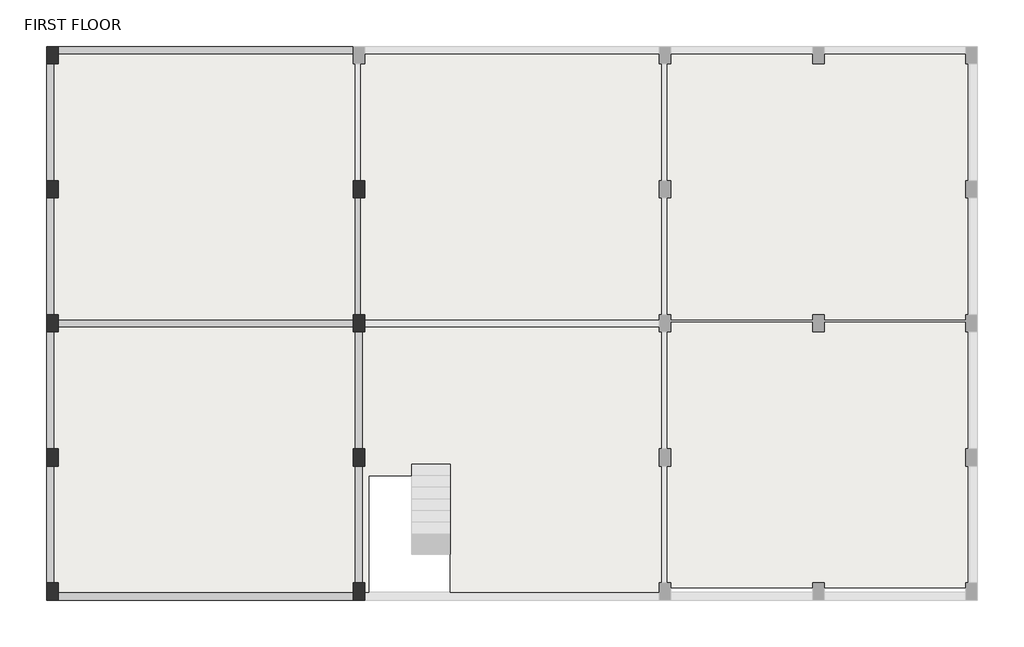
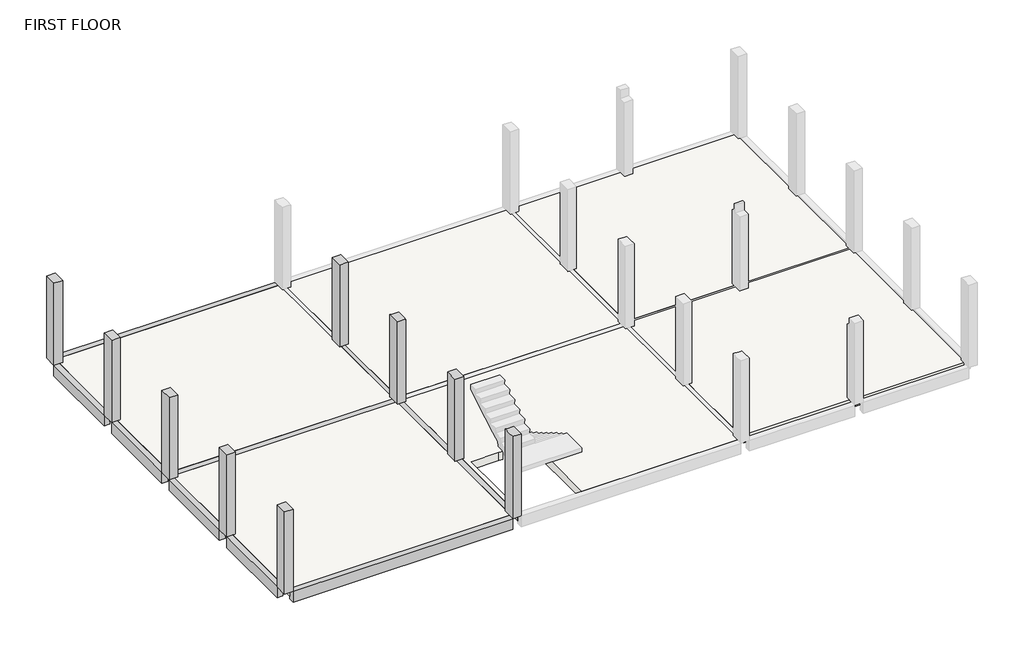
# One storey, part 1 of 2: 10 beams, 9 columns, 1 slab.
"""IFC4 building model written with IfcOpenShell, lengths in millimetres."""

from ifc_helpers import new_model, si_unit, origin, place, context, project, spatial, faceted_brep, element, save

model = new_model("IFC4")

# Units and contexts
model_context = context("Model", 3, world=origin())
ifc_project = project(units=[si_unit("LENGTHUNIT", "METRE", prefix="MILLI")], contexts=[model_context])

# Site, building, storey
site = spatial("IfcSite", under=ifc_project)
building = spatial("IfcBuilding", under=site)
storey = spatial("IfcBuildingStorey", under=building, Name="FIRST FLOOR", Elevation=3048.0)

# Beams
placement = place(None, origin())
element("IfcBeam", 1, ObjectType="M_Concrete-Rectangular Beam : 200MMX400MM", at=placement, inside=storey, context=model_context, shape_type="Brep", body=[
    faceted_brep([(-3980.6874017, 15797.7008557, 3048.0), (-3980.6874017, 15997.7008557, 3048.0), (-11680.6874017, 15997.7008557, 3048.0), (-11680.6874017, 15797.7008557, 3048.0), (-3980.6874017, 15797.7008557, 2648.0), (-3980.6874017, 15797.7008557, 2748.0), (-11680.6874017, 15797.7008557, 2748.0), (-11680.6874017, 15797.7008557, 2648.0), (-3980.6874017, 15997.7008557, 2648.0), (-11680.6874017, 15997.7008557, 2648.0)], [[[0, 1, 2, 3]], [[4, 5, 0, 3, 6, 7]], [[8, 4, 7, 9]], [[1, 8, 9, 2]], [[2, 9, 7, 6, 3]], [[1, 0, 5, 4, 8]]]),
])
element("IfcBeam", 2, ObjectType="M_Concrete-Rectangular Beam : 200MMX400MM", at=placement, inside=storey, context=model_context, shape_type="Brep", body=[
    faceted_brep([(-11680.6874017, 1747.7008557, 3048.0), (-11680.6874017, 1547.7008557, 3048.0), (-3980.6874017, 1547.7008557, 3048.0), (-3980.6874017, 1747.7008557, 3048.0), (-11680.6874017, 1747.7008557, 2648.0), (-11680.6874017, 1747.7008557, 2748.0), (-3980.6874017, 1747.7008557, 2748.0), (-3980.6874017, 1747.7008557, 2648.0), (-11680.6874017, 1547.7008557, 2648.0), (-3980.6874017, 1547.7008557, 2648.0)], [[[0, 1, 2, 3]], [[4, 5, 0, 3, 6, 7]], [[8, 4, 7, 9]], [[1, 8, 9, 2]], [[1, 0, 5, 4, 8]], [[2, 9, 7, 6, 3]]]),
])
element("IfcBeam", 3, ObjectType="M_Concrete-Rectangular Beam : 200MMX400MM", at=placement, inside=storey, context=model_context, shape_type="Brep", body=[
    faceted_brep([(-3980.6874017, 8872.7008557, 3048.0), (-11680.6874017, 8872.7008557, 3048.0), (-11680.6874017, 8672.7008557, 3048.0), (-3980.6874017, 8672.7008557, 3048.0), (-11680.6874017, 8672.7008557, 2748.0), (-11680.6874017, 8672.7008557, 2648.0), (-3980.6874017, 8672.7008557, 2648.0), (-3980.6874017, 8672.7008557, 2748.0), (-11680.6874017, 8872.7008557, 2648.0), (-3980.6874017, 8872.7008557, 2648.0), (-3980.6874017, 8872.7008557, 2748.0), (-11680.6874017, 8872.7008557, 2748.0)], [[[0, 1, 2, 3]], [[3, 2, 4, 5, 6, 7]], [[6, 5, 8, 9]], [[1, 0, 10, 9, 8, 11]], [[8, 5, 4, 2, 1, 11]], [[0, 3, 7, 6, 9, 10]]]),
])
element("IfcBeam", 4, ObjectType="M_Concrete-Rectangular Beam : 200MMX400MM", at=placement, inside=storey, context=model_context, shape_type="Brep", body=[
    faceted_brep([(-11980.6874017, 12497.7008557, 3048.0), (-11780.6874017, 12497.7008557, 3048.0), (-11780.6874017, 15547.7008557, 3048.0), (-11980.6874017, 15547.7008557, 3048.0), (-11980.6874017, 12497.7008557, 2648.0), (-11980.6874017, 15547.7008557, 2648.0), (-11780.6874017, 12497.7008557, 2648.0), (-11780.6874017, 15547.7008557, 2648.0), (-11780.6874017, 12497.7008557, 2748.0), (-11780.6874017, 15547.7008557, 2748.0)], [[[0, 1, 2, 3]], [[4, 0, 3, 5]], [[6, 4, 5, 7]], [[1, 8, 6, 7, 9, 2]], [[2, 9, 7, 5, 3]], [[1, 0, 4, 6, 8]]]),
])
element("IfcBeam", 5, ObjectType="M_Concrete-Rectangular Beam : 200MMX400MM", at=placement, inside=storey, context=model_context, shape_type="Brep", body=[
    faceted_brep([(-11980.6874017, 8997.7008557, 3048.0), (-11780.6874017, 8997.7008557, 3048.0), (-11780.6874017, 12047.7008557, 3048.0), (-11980.6874017, 12047.7008557, 3048.0), (-11980.6874017, 8997.7008557, 2648.0), (-11980.6874017, 12047.7008557, 2648.0), (-11780.6874017, 8997.7008557, 2648.0), (-11780.6874017, 12047.7008557, 2648.0), (-11780.6874017, 8997.7008557, 2748.0), (-11780.6874017, 12047.7008557, 2748.0)], [[[0, 1, 2, 3]], [[4, 0, 3, 5]], [[6, 4, 5, 7]], [[1, 8, 6, 7, 9, 2]], [[1, 0, 4, 6, 8]], [[2, 9, 7, 5, 3]]]),
])
element("IfcBeam", 6, ObjectType="M_Concrete-Rectangular Beam : 200MMX400MM", at=placement, inside=storey, context=model_context, shape_type="Brep", body=[
    faceted_brep([(-11980.6874017, 5497.7008557, 3048.0), (-11780.6874017, 5497.7008557, 3048.0), (-11780.6874017, 8547.7008557, 3048.0), (-11980.6874017, 8547.7008557, 3048.0), (-11980.6874017, 5497.7008557, 2648.0), (-11980.6874017, 8547.7008557, 2648.0), (-11780.6874017, 5497.7008557, 2648.0), (-11780.6874017, 8547.7008557, 2648.0), (-11780.6874017, 5497.7008557, 2748.0), (-11780.6874017, 8547.7008557, 2748.0)], [[[0, 1, 2, 3]], [[4, 0, 3, 5]], [[6, 4, 5, 7]], [[1, 8, 6, 7, 9, 2]], [[2, 9, 7, 5, 3]], [[1, 0, 4, 6, 8]]]),
])
element("IfcBeam", 7, ObjectType="M_Concrete-Rectangular Beam : 200MMX400MM", at=placement, inside=storey, context=model_context, shape_type="Brep", body=[
    faceted_brep([(-11980.6874017, 1997.7008557, 3048.0), (-11780.6874017, 1997.7008557, 3048.0), (-11780.6874017, 5047.7008557, 3048.0), (-11980.6874017, 5047.7008557, 3048.0), (-11980.6874017, 1997.7008557, 2648.0), (-11980.6874017, 5047.7008557, 2648.0), (-11780.6874017, 1997.7008557, 2648.0), (-11780.6874017, 5047.7008557, 2648.0), (-11780.6874017, 1997.7008557, 2748.0), (-11780.6874017, 5047.7008557, 2748.0)], [[[0, 1, 2, 3]], [[4, 0, 3, 5]], [[6, 4, 5, 7]], [[1, 8, 6, 7, 9, 2]], [[1, 0, 4, 6, 8]], [[2, 9, 7, 5, 3]]]),
])
element("IfcBeam", 8, ObjectType="M_Concrete-Rectangular Beam : 200MMX400MM", at=placement, inside=storey, context=model_context, shape_type="Brep", body=[
    faceted_brep([(-3930.6874017, 5047.7008557, 3048.0), (-3930.6874017, 1997.7008557, 3048.0), (-3730.6874017, 1997.7008557, 3048.0), (-3730.6874017, 5047.7008557, 3048.0), (-3730.6874017, 1997.7008557, 2748.0), (-3730.6874017, 1997.7008557, 2648.0), (-3730.6874017, 5047.7008557, 2648.0), (-3730.6874017, 5047.7008557, 2748.0), (-3930.6874017, 1997.7008557, 2648.0), (-3930.6874017, 5047.7008557, 2648.0), (-3930.6874017, 5047.7008557, 2748.0), (-3930.6874017, 1997.7008557, 2748.0)], [[[0, 1, 2, 3]], [[3, 2, 4, 5, 6, 7]], [[6, 5, 8, 9]], [[1, 0, 10, 9, 8, 11]], [[8, 5, 4, 2, 1, 11]], [[0, 3, 7, 6, 9, 10]]]),
])
element("IfcBeam", 9, ObjectType="M_Concrete-Rectangular Beam : 200MMX400MM", at=placement, inside=storey, context=model_context, shape_type="Brep", body=[
    faceted_brep([(-3930.6874017, 8547.7008557, 3048.0), (-3930.6874017, 5497.7008557, 3048.0), (-3730.6874017, 5497.7008557, 3048.0), (-3730.6874017, 8547.7008557, 3048.0), (-3730.6874017, 5497.7008557, 2748.0), (-3730.6874017, 5497.7008557, 2648.0), (-3730.6874017, 8547.7008557, 2648.0), (-3730.6874017, 8547.7008557, 2748.0), (-3930.6874017, 5497.7008557, 2648.0), (-3930.6874017, 8547.7008557, 2648.0), (-3930.6874017, 8547.7008557, 2748.0), (-3930.6874017, 5497.7008557, 2748.0)], [[[0, 1, 2, 3]], [[3, 2, 4, 5, 6, 7]], [[6, 5, 8, 9]], [[1, 0, 10, 9, 8, 11]], [[0, 3, 7, 6, 9, 10]], [[8, 5, 4, 2, 1, 11]]]),
])
element("IfcBeam", 10, ObjectType="M_Concrete-Rectangular Beam : 200MMX400MM", at=placement, inside=storey, context=model_context, shape_type="Brep", body=[
    faceted_brep([(-3930.6874017, 12047.7008557, 3048.0), (-3930.6874017, 8997.7008557, 3048.0), (-3780.6874017, 8997.7008557, 3048.0), (-3780.6874017, 12047.7008557, 3048.0), (-3730.6874017, 8997.7008557, 2648.0), (-3730.6874017, 12047.7008557, 2648.0), (-3730.6874017, 12047.7008557, 2748.0), (-3730.6874017, 8997.7008557, 2748.0), (-3930.6874017, 8997.7008557, 2648.0), (-3930.6874017, 12047.7008557, 2648.0), (-3930.6874017, 12047.7008557, 2748.0), (-3930.6874017, 8997.7008557, 2748.0), (-3780.6874017, 12047.7008557, 2748.0), (-3780.6874017, 8997.7008557, 2748.0)], [[[0, 1, 2, 3]], [[4, 5, 6, 7]], [[5, 4, 8, 9]], [[1, 0, 10, 9, 8, 11]], [[5, 9, 10, 0, 3, 12, 6]], [[8, 4, 7, 13, 2, 1, 11]], [[12, 13, 7, 6]], [[13, 12, 3, 2]]]),
])

# Columns
element("IfcColumn", 11, ObjectType="M_Concrete-Rectangular-Column : 300 x 450mm", at=placement, inside=storey, context=model_context, shape_type="Brep", body=[
    faceted_brep([(-11680.6874017, 15997.7008557, 3048.0), (-11680.6874017, 15547.7008557, 3048.0), (-11980.6874017, 15547.7008557, 3048.0), (-11980.6874017, 15997.7008557, 3048.0), (-11680.6874017, 15997.7008557, 6096.0), (-11680.6874017, 15797.7008557, 6096.0), (-11680.6874017, 15547.7008557, 6096.0), (-11680.6874017, 15547.7008557, 5796.0), (-11780.6874017, 15547.7008557, 6096.0), (-11980.6874017, 15547.7008557, 6096.0), (-11980.6874017, 15997.7008557, 6096.0)], [[[0, 1, 2, 3]], [[1, 0, 4, 5, 6, 7]], [[2, 1, 7, 6, 8, 9]], [[3, 2, 9, 10]], [[0, 3, 10, 4]], [[10, 9, 8, 6, 5, 4]]]),
])
element("IfcColumn", 12, ObjectType="M_Concrete-Rectangular-Column : 300 x 450mm", at=placement, inside=storey, context=model_context, shape_type="Brep", body=[
    faceted_brep([(-11680.6874017, 8997.7008557, 3048.0), (-11680.6874017, 8547.7008557, 3048.0), (-11980.6874017, 8547.7008557, 3048.0), (-11980.6874017, 8997.7008557, 3048.0), (-11680.6874017, 8997.7008557, 5796.0), (-11680.6874017, 8997.7008557, 6096.0), (-11680.6874017, 8872.7008557, 6096.0), (-11680.6874017, 8672.7008557, 6096.0), (-11680.6874017, 8547.7008557, 6096.0), (-11680.6874017, 8547.7008557, 5796.0), (-11780.6874017, 8547.7008557, 6096.0), (-11980.6874017, 8547.7008557, 6096.0), (-11980.6874017, 8997.7008557, 6096.0), (-11780.6874017, 8997.7008557, 6096.0)], [[[0, 1, 2, 3]], [[1, 0, 4, 5, 6, 7, 8, 9]], [[2, 1, 9, 8, 10, 11]], [[3, 2, 11, 12]], [[0, 3, 12, 13, 5, 4]], [[12, 11, 10, 8, 7, 6, 5, 13]]]),
])
element("IfcColumn", 13, ObjectType="M_Concrete-Rectangular-Column : 300 x 450mm", at=placement, inside=storey, context=model_context, shape_type="Brep", body=[
    faceted_brep([(-11680.6874017, 1997.7008557, 3048.0), (-11680.6874017, 1547.7008557, 3048.0), (-11980.6874017, 1547.7008557, 3048.0), (-11980.6874017, 1997.7008557, 3048.0), (-11680.6874017, 1997.7008557, 5796.0), (-11680.6874017, 1997.7008557, 6096.0), (-11680.6874017, 1747.7008557, 6096.0), (-11680.6874017, 1547.7008557, 6096.0), (-11980.6874017, 1547.7008557, 6096.0), (-11980.6874017, 1997.7008557, 6096.0), (-11780.6874017, 1997.7008557, 6096.0)], [[[0, 1, 2, 3]], [[1, 0, 4, 5, 6, 7]], [[2, 1, 7, 8]], [[3, 2, 8, 9]], [[0, 3, 9, 10, 5, 4]], [[8, 7, 6, 5, 10, 9]]]),
])
element("IfcColumn", 14, ObjectType="M_Concrete-Rectangular-Column : 300 x 450mm", at=placement, inside=storey, context=model_context, shape_type="Brep", body=[
    faceted_brep([(-3680.6874017, 12497.7008557, 3048.0), (-3680.6874017, 12047.7008557, 3048.0), (-3980.6874017, 12047.7008557, 3048.0), (-3980.6874017, 12497.7008557, 3048.0), (-3680.6874017, 12497.7008557, 5796.0), (-3680.6874017, 12497.7008557, 6096.0), (-3680.6874017, 12047.7008557, 6096.0), (-3680.6874017, 12047.7008557, 5796.0), (-3780.6874017, 12047.7008557, 6096.0), (-3930.6874017, 12047.7008557, 6096.0), (-3980.6874017, 12047.7008557, 6096.0), (-3980.6874017, 12047.7008557, 5796.0), (-3980.6874017, 12497.7008557, 6096.0), (-3980.6874017, 12497.7008557, 5796.0), (-3930.6874017, 12497.7008557, 6096.0), (-3780.6874017, 12497.7008557, 6096.0)], [[[0, 1, 2, 3]], [[1, 0, 4, 5, 6, 7]], [[2, 1, 7, 6, 8, 9, 10, 11]], [[3, 2, 11, 10, 12, 13]], [[0, 3, 13, 12, 14, 15, 5, 4]], [[6, 5, 15, 14, 12, 10, 9, 8]]]),
])
element("IfcColumn", 15, ObjectType="M_Concrete-Rectangular-Column : 300 x 450mm", at=placement, inside=storey, context=model_context, shape_type="Brep", body=[
    faceted_brep([(-3680.6874017, 8997.7008557, 3048.0), (-3680.6874017, 8547.7008557, 3048.0), (-3980.6874017, 8547.7008557, 3048.0), (-3980.6874017, 8997.7008557, 3048.0), (-3680.6874017, 8997.7008557, 5796.0), (-3680.6874017, 8997.7008557, 6096.0), (-3680.6874017, 8872.7008557, 6096.0), (-3680.6874017, 8672.7008557, 6096.0), (-3680.6874017, 8547.7008557, 6096.0), (-3680.6874017, 8547.7008557, 5796.0), (-3730.6874017, 8547.7008557, 6096.0), (-3930.6874017, 8547.7008557, 6096.0), (-3980.6874017, 8547.7008557, 6096.0), (-3980.6874017, 8547.7008557, 5796.0), (-3980.6874017, 8672.7008557, 6096.0), (-3980.6874017, 8872.7008557, 6096.0), (-3980.6874017, 8997.7008557, 6096.0), (-3980.6874017, 8997.7008557, 5796.0), (-3930.6874017, 8997.7008557, 6096.0), (-3780.6874017, 8997.7008557, 6096.0)], [[[0, 1, 2, 3]], [[1, 0, 4, 5, 6, 7, 8, 9]], [[2, 1, 9, 8, 10, 11, 12, 13]], [[3, 2, 13, 12, 14, 15, 16, 17]], [[0, 3, 17, 16, 18, 19, 5, 4]], [[18, 16, 15, 14, 12, 11, 10, 8, 7, 6, 5, 19]]]),
])
element("IfcColumn", 16, ObjectType="M_Concrete-Rectangular-Column : 300 x 450mm", at=placement, inside=storey, context=model_context, shape_type="Brep", body=[
    faceted_brep([(-3680.6874017, 5497.7008557, 3048.0), (-3680.6874017, 5047.7008557, 3048.0), (-3980.6874017, 5047.7008557, 3048.0), (-3980.6874017, 5497.7008557, 3048.0), (-3680.6874017, 5497.7008557, 5796.0), (-3680.6874017, 5497.7008557, 6096.0), (-3680.6874017, 5047.7008557, 6096.0), (-3680.6874017, 5047.7008557, 5796.0), (-3730.6874017, 5047.7008557, 6096.0), (-3930.6874017, 5047.7008557, 6096.0), (-3980.6874017, 5047.7008557, 6096.0), (-3980.6874017, 5047.7008557, 5796.0), (-3980.6874017, 5497.7008557, 6096.0), (-3980.6874017, 5497.7008557, 5796.0), (-3930.6874017, 5497.7008557, 6096.0), (-3730.6874017, 5497.7008557, 6096.0)], [[[0, 1, 2, 3]], [[1, 0, 4, 5, 6, 7]], [[2, 1, 7, 6, 8, 9, 10, 11]], [[3, 2, 11, 10, 12, 13]], [[0, 3, 13, 12, 14, 15, 5, 4]], [[6, 5, 15, 14, 12, 10, 9, 8]]]),
])
element("IfcColumn", 17, ObjectType="M_Concrete-Rectangular-Column : 300 x 450mm", at=placement, inside=storey, context=model_context, shape_type="Brep", body=[
    faceted_brep([(-3680.6874017, 1997.7008557, 3048.0), (-3680.6874017, 1547.7008557, 3048.0), (-3980.6874017, 1547.7008557, 3048.0), (-3980.6874017, 1997.7008557, 3048.0), (-3680.6874017, 1997.7008557, 5796.0), (-3680.6874017, 1997.7008557, 6096.0), (-3680.6874017, 1747.7008557, 6096.0), (-3680.6874017, 1547.7008557, 6096.0), (-3980.6874017, 1547.7008557, 6096.0), (-3980.6874017, 1747.7008557, 6096.0), (-3980.6874017, 1997.7008557, 6096.0), (-3980.6874017, 1997.7008557, 5796.0), (-3930.6874017, 1997.7008557, 6096.0), (-3730.6874017, 1997.7008557, 6096.0)], [[[0, 1, 2, 3]], [[1, 0, 4, 5, 6, 7]], [[2, 1, 7, 8]], [[3, 2, 8, 9, 10, 11]], [[0, 3, 11, 10, 12, 13, 5, 4]], [[8, 7, 6, 5, 13, 12, 10, 9]]]),
])
element("IfcColumn", 18, ObjectType="M_Concrete-Rectangular-Column : 300 x 450mm", at=placement, inside=storey, context=model_context, shape_type="Brep", body=[
    faceted_brep([(-11680.6874017, 12497.7008557, 3048.0), (-11680.6874017, 12047.7008557, 3048.0), (-11980.6874017, 12047.7008557, 3048.0), (-11980.6874017, 12497.7008557, 3048.0), (-11680.6874017, 12497.7008557, 5796.0), (-11680.6874017, 12497.7008557, 6096.0), (-11680.6874017, 12047.7008557, 6096.0), (-11680.6874017, 12047.7008557, 5796.0), (-11780.6874017, 12047.7008557, 6096.0), (-11980.6874017, 12047.7008557, 6096.0), (-11980.6874017, 12497.7008557, 6096.0), (-11780.6874017, 12497.7008557, 6096.0)], [[[0, 1, 2, 3]], [[1, 0, 4, 5, 6, 7]], [[2, 1, 7, 6, 8, 9]], [[3, 2, 9, 10]], [[0, 3, 10, 11, 5, 4]], [[6, 5, 11, 10, 9, 8]]]),
])
element("IfcColumn", 19, ObjectType="M_Concrete-Rectangular-Column : 300 x 450mm", at=placement, inside=storey, context=model_context, shape_type="Brep", body=[
    faceted_brep([(-11680.6874017, 5497.7008557, 3048.0), (-11680.6874017, 5047.7008557, 3048.0), (-11980.6874017, 5047.7008557, 3048.0), (-11980.6874017, 5497.7008557, 3048.0), (-11680.6874017, 5497.7008557, 5796.0), (-11680.6874017, 5497.7008557, 6096.0), (-11680.6874017, 5047.7008557, 6096.0), (-11680.6874017, 5047.7008557, 5796.0), (-11780.6874017, 5047.7008557, 6096.0), (-11980.6874017, 5047.7008557, 6096.0), (-11980.6874017, 5497.7008557, 6096.0), (-11780.6874017, 5497.7008557, 6096.0)], [[[0, 1, 2, 3]], [[1, 0, 4, 5, 6, 7]], [[2, 1, 7, 6, 8, 9]], [[3, 2, 9, 10]], [[0, 3, 10, 11, 5, 4]], [[6, 5, 11, 10, 9, 8]]]),
])

# Slab
element("IfcSlab", 20, ObjectType="Generic 300mm", at=placement, inside=storey, context=model_context, shape_type="Brep", body=[
    faceted_brep([(-11680.6874017, 15547.7008557, 2748.0), (-11680.6874017, 15797.7008557, 2748.0), (-3980.6874017, 15797.7008557, 2748.0), (-3980.6874017, 15547.7008557, 2748.0), (-3930.6874017, 15547.7008557, 2748.0), (-3930.6874017, 12497.7008557, 2748.0), (-3980.6874017, 12497.7008557, 2748.0), (-3980.6874017, 12047.7008557, 2748.0), (-3930.6874017, 12047.7008557, 2748.0), (-3930.6874017, 8997.7008557, 2748.0), (-3980.6874017, 8997.7008557, 2748.0), (-3980.6874017, 8872.7008557, 2748.0), (-11680.6874017, 8872.7008557, 2748.0), (-11680.6874017, 8997.7008557, 2748.0), (-11780.6874017, 8997.7008557, 2748.0), (-11780.6874017, 12047.7008557, 2748.0), (-11680.6874017, 12047.7008557, 2748.0), (-11680.6874017, 12497.7008557, 2748.0), (-11780.6874017, 12497.7008557, 2748.0), (-11780.6874017, 15547.7008557, 2748.0), (-11680.6874017, 15797.7008557, 3048.0), (-11680.6874017, 15547.7008557, 3048.0), (-11780.6874017, 15547.7008557, 3048.0), (-11780.6874017, 12497.7008557, 3048.0), (-11680.6874017, 12497.7008557, 3048.0), (-11680.6874017, 12047.7008557, 3048.0), (-11780.6874017, 12047.7008557, 3048.0), (-11780.6874017, 8997.7008557, 3048.0), (-11680.6874017, 8997.7008557, 3048.0), (-11680.6874017, 8872.7008557, 3048.0), (-3980.6874017, 8872.7008557, 3048.0), (-3980.6874017, 8997.7008557, 3048.0), (-3930.6874017, 8997.7008557, 3048.0), (-3930.6874017, 12047.7008557, 3048.0), (-3980.6874017, 12047.7008557, 3048.0), (-3980.6874017, 12497.7008557, 3048.0), (-3930.6874017, 12497.7008557, 3048.0), (-3930.6874017, 15547.7008557, 3048.0), (-3980.6874017, 15547.7008557, 3048.0), (-3980.6874017, 15797.7008557, 3048.0)], [[[0, 1, 2, 3, 4, 5, 6, 7, 8, 9, 10, 11, 12, 13, 14, 15, 16, 17, 18, 19]], [[20, 21, 22, 23, 24, 25, 26, 27, 28, 29, 30, 31, 32, 33, 34, 35, 36, 37, 38, 39]], [[1, 0, 21, 20]], [[2, 1, 20, 39]], [[3, 2, 39, 38]], [[4, 3, 38, 37]], [[5, 4, 37, 36]], [[6, 5, 36, 35]], [[7, 6, 35, 34]], [[8, 7, 34, 33]], [[9, 8, 33, 32]], [[10, 9, 32, 31]], [[11, 10, 31, 30]], [[12, 11, 30, 29]], [[13, 12, 29, 28]], [[14, 13, 28, 27]], [[15, 14, 27, 26]], [[16, 15, 26, 25]], [[17, 16, 25, 24]], [[18, 17, 24, 23]], [[19, 18, 23, 22]], [[0, 19, 22, 21]]]),
    faceted_brep([(-3680.6874017, 15547.7008557, 2748.0), (-3680.6874017, 15797.7008557, 2748.0), (4019.3125983, 15797.7008557, 2748.0), (4019.3125983, 15547.7008557, 2748.0), (4069.3125983, 15547.7008557, 2748.0), (4069.3125983, 12497.7008557, 2748.0), (4019.3125983, 12497.7008557, 2748.0), (4019.3125983, 12047.7008557, 2748.0), (4069.3125983, 12047.7008557, 2748.0), (4069.3125983, 8997.7008557, 2748.0), (4019.3125983, 8997.7008557, 2748.0), (4019.3125983, 8872.7008557, 2748.0), (-3680.6874017, 8872.7008557, 2748.0), (-3680.6874017, 8997.7008557, 2748.0), (-3730.6874017, 8997.7008557, 2748.0), (-3780.6874017, 8997.7008557, 2748.0), (-3780.6874017, 12047.7008557, 2748.0), (-3730.6874017, 12047.7008557, 2748.0), (-3680.6874017, 12047.7008557, 2748.0), (-3680.6874017, 12497.7008557, 2748.0), (-3730.6874017, 12497.7008557, 2748.0), (-3780.6874017, 12497.7008557, 2748.0), (-3780.6874017, 15547.7008557, 2748.0), (-3730.6874017, 15547.7008557, 2748.0), (-3680.6874017, 15797.7008557, 3048.0), (-3680.6874017, 15547.7008557, 3048.0), (-3780.6874017, 15547.7008557, 3048.0), (-3780.6874017, 12497.7008557, 3048.0), (-3680.6874017, 12497.7008557, 3048.0), (-3680.6874017, 12047.7008557, 3048.0), (-3780.6874017, 12047.7008557, 3048.0), (-3780.6874017, 8997.7008557, 3048.0), (-3680.6874017, 8997.7008557, 3048.0), (-3680.6874017, 8872.7008557, 3048.0), (4019.3125983, 8872.7008557, 3048.0), (4019.3125983, 8997.7008557, 3048.0), (4069.3125983, 8997.7008557, 3048.0), (4069.3125983, 12047.7008557, 3048.0), (4019.3125983, 12047.7008557, 3048.0), (4019.3125983, 12497.7008557, 3048.0), (4069.3125983, 12497.7008557, 3048.0), (4069.3125983, 15547.7008557, 3048.0), (4019.3125983, 15547.7008557, 3048.0), (4019.3125983, 15797.7008557, 3048.0)], [[[0, 1, 2, 3, 4, 5, 6, 7, 8, 9, 10, 11, 12, 13, 14, 15, 16, 17, 18, 19, 20, 21, 22, 23]], [[24, 25, 26, 27, 28, 29, 30, 31, 32, 33, 34, 35, 36, 37, 38, 39, 40, 41, 42, 43]], [[1, 0, 25, 24]], [[2, 1, 24, 43]], [[3, 2, 43, 42]], [[4, 3, 42, 41]], [[5, 4, 41, 40]], [[6, 5, 40, 39]], [[7, 6, 39, 38]], [[8, 7, 38, 37]], [[9, 8, 37, 36]], [[10, 9, 36, 35]], [[11, 10, 35, 34]], [[12, 11, 34, 33]], [[13, 12, 33, 32]], [[15, 14, 13, 32, 31]], [[16, 15, 31, 30]], [[18, 17, 16, 30, 29]], [[19, 18, 29, 28]], [[21, 20, 19, 28, 27]], [[22, 21, 27, 26]], [[0, 23, 22, 26, 25]]]),
    faceted_brep([(4319.3125983, 15547.7008557, 2748.0), (4319.3125983, 15797.7008557, 2748.0), (8019.3125983, 15797.7008557, 2748.0), (8319.3125983, 15797.7008557, 2748.0), (12019.3125983, 15797.7008557, 2748.0), (12019.3125983, 15547.7008557, 2748.0), (12069.3125983, 15547.7008557, 2748.0), (12069.3125983, 12497.7008557, 2748.0), (12019.3125983, 12497.7008557, 2748.0), (12019.3125983, 12047.7008557, 2748.0), (12069.3125983, 12047.7008557, 2748.0), (12069.3125983, 8997.7008557, 2748.0), (12019.3125983, 8997.7008557, 2748.0), (12019.3125983, 8872.7008557, 2748.0), (8319.3125983, 8872.7008557, 2748.0), (8019.3125983, 8872.7008557, 2748.0), (4319.3125983, 8872.7008557, 2748.0), (4319.3125983, 8997.7008557, 2748.0), (4269.3125983, 8997.7008557, 2748.0), (4219.3125983, 8997.7008557, 2748.0), (4219.3125983, 12047.7008557, 2748.0), (4269.3125983, 12047.7008557, 2748.0), (4319.3125983, 12047.7008557, 2748.0), (4319.3125983, 12497.7008557, 2748.0), (4269.3125983, 12497.7008557, 2748.0), (4219.3125983, 12497.7008557, 2748.0), (4219.3125983, 15547.7008557, 2748.0), (4269.3125983, 15547.7008557, 2748.0), (4319.3125983, 15797.7008557, 3048.0), (4319.3125983, 15547.7008557, 3048.0), (4219.3125983, 15547.7008557, 3048.0), (4219.3125983, 12497.7008557, 3048.0), (4319.3125983, 12497.7008557, 3048.0), (4319.3125983, 12047.7008557, 3048.0), (4219.3125983, 12047.7008557, 3048.0), (4219.3125983, 8997.7008557, 3048.0), (4319.3125983, 8997.7008557, 3048.0), (4319.3125983, 8872.7008557, 3048.0), (8019.3125983, 8872.7008557, 3048.0), (8319.3125983, 8872.7008557, 3048.0), (12019.3125983, 8872.7008557, 3048.0), (12019.3125983, 8997.7008557, 3048.0), (12069.3125983, 8997.7008557, 3048.0), (12069.3125983, 12047.7008557, 3048.0), (12019.3125983, 12047.7008557, 3048.0), (12019.3125983, 12497.7008557, 3048.0), (12069.3125983, 12497.7008557, 3048.0), (12069.3125983, 15547.7008557, 3048.0), (12019.3125983, 15547.7008557, 3048.0), (12019.3125983, 15797.7008557, 3048.0), (8319.3125983, 15797.7008557, 3048.0), (8019.3125983, 15797.7008557, 3048.0)], [[[0, 1, 2, 3, 4, 5, 6, 7, 8, 9, 10, 11, 12, 13, 14, 15, 16, 17, 18, 19, 20, 21, 22, 23, 24, 25, 26, 27]], [[28, 29, 30, 31, 32, 33, 34, 35, 36, 37, 38, 39, 40, 41, 42, 43, 44, 45, 46, 47, 48, 49, 50, 51]], [[1, 0, 29, 28]], [[4, 3, 2, 1, 28, 51, 50, 49]], [[5, 4, 49, 48]], [[6, 5, 48, 47]], [[7, 6, 47, 46]], [[8, 7, 46, 45]], [[9, 8, 45, 44]], [[10, 9, 44, 43]], [[11, 10, 43, 42]], [[12, 11, 42, 41]], [[13, 12, 41, 40]], [[16, 15, 14, 13, 40, 39, 38, 37]], [[17, 16, 37, 36]], [[19, 18, 17, 36, 35]], [[20, 19, 35, 34]], [[22, 21, 20, 34, 33]], [[23, 22, 33, 32]], [[25, 24, 23, 32, 31]], [[26, 25, 31, 30]], [[0, 27, 26, 30, 29]]]),
    faceted_brep([(-3680.6874017, 8547.7008557, 2748.0), (-3680.6874017, 8672.7008557, 2748.0), (4019.3125983, 8672.7008557, 2748.0), (4019.3125983, 8547.7008557, 2748.0), (4069.3125983, 8547.7008557, 2748.0), (4069.3125983, 5497.7008557, 2748.0), (4019.3125983, 5497.7008557, 2748.0), (4019.3125983, 5047.7008557, 2748.0), (4069.3125983, 5047.7008557, 2748.0), (4069.3125983, 1997.7008557, 2748.0), (4019.3125983, 1997.7008557, 2748.0), (4019.3125983, 1747.7008557, 2748.0), (-1437.0874017, 1747.7008557, 2748.0), (-1437.0874017, 5100.5008557, 2748.0), (-2453.0874017, 5100.5008557, 2748.0), (-2453.0874017, 4795.7008557, 2748.0), (-2593.0874017, 4795.7008557, 2748.0), (-3570.6874017, 4795.7008557, 2748.0), (-3570.6874017, 1747.7008557, 2748.0), (-3680.6874017, 1747.7008557, 2748.0), (-3680.6874017, 1997.7008557, 2748.0), (-3730.6874017, 1997.7008557, 2748.0), (-3730.6874017, 5047.7008557, 2748.0), (-3680.6874017, 5047.7008557, 2748.0), (-3680.6874017, 5497.7008557, 2748.0), (-3730.6874017, 5497.7008557, 2748.0), (-3730.6874017, 8547.7008557, 2748.0), (-3680.6874017, 8672.7008557, 3048.0), (-3680.6874017, 8547.7008557, 3048.0), (-3730.6874017, 8547.7008557, 3048.0), (-3730.6874017, 5497.7008557, 3048.0), (-3680.6874017, 5497.7008557, 3048.0), (-3680.6874017, 5047.7008557, 3048.0), (-3730.6874017, 5047.7008557, 3048.0), (-3730.6874017, 1997.7008557, 3048.0), (-3680.6874017, 1997.7008557, 3048.0), (-3680.6874017, 1747.7008557, 3048.0), (-3570.6874017, 1747.7008557, 3048.0), (-3570.6874017, 4795.7008557, 3048.0), (-2593.0874017, 4795.7008557, 3048.0), (-2453.0874017, 4795.7008557, 3048.0), (-2453.0874017, 5100.5008557, 3048.0), (-1437.0874017, 5100.5008557, 3048.0), (-1437.0874017, 1747.7008557, 3048.0), (4019.3125983, 1747.7008557, 3048.0), (4019.3125983, 1997.7008557, 3048.0), (4069.3125983, 1997.7008557, 3048.0), (4069.3125983, 5047.7008557, 3048.0), (4019.3125983, 5047.7008557, 3048.0), (4019.3125983, 5497.7008557, 3048.0), (4069.3125983, 5497.7008557, 3048.0), (4069.3125983, 8547.7008557, 3048.0), (4019.3125983, 8547.7008557, 3048.0), (4019.3125983, 8672.7008557, 3048.0)], [[[0, 1, 2, 3, 4, 5, 6, 7, 8, 9, 10, 11, 12, 13, 14, 15, 16, 17, 18, 19, 20, 21, 22, 23, 24, 25, 26]], [[27, 28, 29, 30, 31, 32, 33, 34, 35, 36, 37, 38, 39, 40, 41, 42, 43, 44, 45, 46, 47, 48, 49, 50, 51, 52, 53]], [[1, 0, 28, 27]], [[2, 1, 27, 53]], [[3, 2, 53, 52]], [[4, 3, 52, 51]], [[5, 4, 51, 50]], [[6, 5, 50, 49]], [[7, 6, 49, 48]], [[8, 7, 48, 47]], [[9, 8, 47, 46]], [[10, 9, 46, 45]], [[11, 10, 45, 44]], [[11, 44, 43, 12]], [[36, 19, 18, 37]], [[20, 19, 36, 35]], [[21, 20, 35, 34]], [[22, 21, 34, 33]], [[23, 22, 33, 32]], [[24, 23, 32, 31]], [[25, 24, 31, 30]], [[26, 25, 30, 29]], [[0, 26, 29, 28]], [[42, 13, 12, 43]], [[13, 42, 41, 14]], [[14, 41, 40, 15]], [[15, 40, 39, 16]], [[16, 39, 38, 17]], [[17, 38, 37, 18]]]),
    faceted_brep([(-3980.6874017, 1747.7008557, 2748.0), (-11680.6874017, 1747.7008557, 2748.0), (-11680.6874017, 1997.7008557, 2748.0), (-11780.6874017, 1997.7008557, 2748.0), (-11780.6874017, 5047.7008557, 2748.0), (-11680.6874017, 5047.7008557, 2748.0), (-11680.6874017, 5497.7008557, 2748.0), (-11780.6874017, 5497.7008557, 2748.0), (-11780.6874017, 8547.7008557, 2748.0), (-11680.6874017, 8547.7008557, 2748.0), (-11680.6874017, 8672.7008557, 2748.0), (-3980.6874017, 8672.7008557, 2748.0), (-3980.6874017, 8547.7008557, 2748.0), (-3930.6874017, 8547.7008557, 2748.0), (-3930.6874017, 5497.7008557, 2748.0), (-3980.6874017, 5497.7008557, 2748.0), (-3980.6874017, 5047.7008557, 2748.0), (-3930.6874017, 5047.7008557, 2748.0), (-3930.6874017, 1997.7008557, 2748.0), (-3980.6874017, 1997.7008557, 2748.0), (-11680.6874017, 1747.7008557, 3048.0), (-3980.6874017, 1747.7008557, 3048.0), (-3980.6874017, 1997.7008557, 3048.0), (-3930.6874017, 1997.7008557, 3048.0), (-3930.6874017, 5047.7008557, 3048.0), (-3980.6874017, 5047.7008557, 3048.0), (-3980.6874017, 5497.7008557, 3048.0), (-3930.6874017, 5497.7008557, 3048.0), (-3930.6874017, 8547.7008557, 3048.0), (-3980.6874017, 8547.7008557, 3048.0), (-3980.6874017, 8672.7008557, 3048.0), (-11680.6874017, 8672.7008557, 3048.0), (-11680.6874017, 8547.7008557, 3048.0), (-11780.6874017, 8547.7008557, 3048.0), (-11780.6874017, 5497.7008557, 3048.0), (-11680.6874017, 5497.7008557, 3048.0), (-11680.6874017, 5047.7008557, 3048.0), (-11780.6874017, 5047.7008557, 3048.0), (-11780.6874017, 1997.7008557, 3048.0), (-11680.6874017, 1997.7008557, 3048.0)], [[[0, 1, 2, 3, 4, 5, 6, 7, 8, 9, 10, 11, 12, 13, 14, 15, 16, 17, 18, 19]], [[20, 21, 22, 23, 24, 25, 26, 27, 28, 29, 30, 31, 32, 33, 34, 35, 36, 37, 38, 39]], [[1, 0, 21, 20]], [[2, 1, 20, 39]], [[3, 2, 39, 38]], [[4, 3, 38, 37]], [[5, 4, 37, 36]], [[6, 5, 36, 35]], [[7, 6, 35, 34]], [[8, 7, 34, 33]], [[9, 8, 33, 32]], [[10, 9, 32, 31]], [[11, 10, 31, 30]], [[12, 11, 30, 29]], [[13, 12, 29, 28]], [[14, 13, 28, 27]], [[15, 14, 27, 26]], [[16, 15, 26, 25]], [[17, 16, 25, 24]], [[18, 17, 24, 23]], [[19, 18, 23, 22]], [[0, 19, 22, 21]]]),
    faceted_brep([(4319.3125983, 8547.7008557, 2748.0), (4319.3125983, 8672.7008557, 2748.0), (4319.3125983, 8797.7008557, 2748.0), (8019.3125983, 8797.7008557, 2748.0), (8319.3125983, 8797.7008557, 2748.0), (12019.3125983, 8797.7008557, 2748.0), (12019.3125983, 8672.7008557, 2748.0), (12019.3125983, 8547.7008557, 2748.0), (12069.3125983, 8547.7008557, 2748.0), (12069.3125983, 5497.7008557, 2748.0), (12019.3125983, 5497.7008557, 2748.0), (12019.3125983, 5047.7008557, 2748.0), (12069.3125983, 5047.7008557, 2748.0), (12069.3125983, 1997.7008557, 2748.0), (12019.3125983, 1997.7008557, 2748.0), (12019.3125983, 1872.7008557, 2748.0), (8319.3125983, 1872.7008557, 2748.0), (8019.3125983, 1872.7008557, 2748.0), (4319.3125983, 1872.7008557, 2748.0), (4319.3125983, 1997.7008557, 2748.0), (4269.3125983, 1997.7008557, 2748.0), (4219.3125983, 1997.7008557, 2748.0), (4219.3125983, 5047.7008557, 2748.0), (4269.3125983, 5047.7008557, 2748.0), (4319.3125983, 5047.7008557, 2748.0), (4319.3125983, 5497.7008557, 2748.0), (4269.3125983, 5497.7008557, 2748.0), (4219.3125983, 5497.7008557, 2748.0), (4219.3125983, 8547.7008557, 2748.0), (4269.3125983, 8547.7008557, 2748.0), (4319.3125983, 8797.7008557, 3048.0), (4319.3125983, 8547.7008557, 3048.0), (4219.3125983, 8547.7008557, 3048.0), (4219.3125983, 5497.7008557, 3048.0), (4319.3125983, 5497.7008557, 3048.0), (4319.3125983, 5047.7008557, 3048.0), (4219.3125983, 5047.7008557, 3048.0), (4219.3125983, 1997.7008557, 3048.0), (4319.3125983, 1997.7008557, 3048.0), (4319.3125983, 1872.7008557, 3048.0), (8019.3125983, 1872.7008557, 3048.0), (8319.3125983, 1872.7008557, 3048.0), (12019.3125983, 1872.7008557, 3048.0), (12019.3125983, 1997.7008557, 3048.0), (12069.3125983, 1997.7008557, 3048.0), (12069.3125983, 5047.7008557, 3048.0), (12019.3125983, 5047.7008557, 3048.0), (12019.3125983, 5497.7008557, 3048.0), (12069.3125983, 5497.7008557, 3048.0), (12069.3125983, 8547.7008557, 3048.0), (12019.3125983, 8547.7008557, 3048.0), (12019.3125983, 8797.7008557, 3048.0), (8319.3125983, 8797.7008557, 3048.0), (8019.3125983, 8797.7008557, 3048.0)], [[[0, 1, 2, 3, 4, 5, 6, 7, 8, 9, 10, 11, 12, 13, 14, 15, 16, 17, 18, 19, 20, 21, 22, 23, 24, 25, 26, 27, 28, 29]], [[30, 31, 32, 33, 34, 35, 36, 37, 38, 39, 40, 41, 42, 43, 44, 45, 46, 47, 48, 49, 50, 51, 52, 53]], [[2, 1, 0, 31, 30]], [[5, 4, 3, 2, 30, 53, 52, 51]], [[7, 6, 5, 51, 50]], [[8, 7, 50, 49]], [[9, 8, 49, 48]], [[10, 9, 48, 47]], [[11, 10, 47, 46]], [[12, 11, 46, 45]], [[13, 12, 45, 44]], [[14, 13, 44, 43]], [[15, 14, 43, 42]], [[18, 17, 16, 15, 42, 41, 40, 39]], [[19, 18, 39, 38]], [[21, 20, 19, 38, 37]], [[22, 21, 37, 36]], [[24, 23, 22, 36, 35]], [[25, 24, 35, 34]], [[27, 26, 25, 34, 33]], [[28, 27, 33, 32]], [[0, 29, 28, 32, 31]]]),
])

save(model, "model.ifc")

# Revit data of these elements
# Type "M_Concrete-Rectangular Beam : 200MMX400MM"
#   Length [instance default] = 5' - 0"
#   b = 0' - 7.87402"
#   h = 1' - 3.74803"
#   Structural Material [instance default] = Concrete, Cast-in-Place gray
#   Assembly Code = ""
# Type "M_Concrete-Rectangular-Column : 300 x 450mm"
#   b = 0' - 11.81102"
#   h = 1' - 5.71654"
#   Structural Material [instance default] = Concrete, Cast-in-Place gray
# Type "Generic 300mm"
#   Function = 0
#   Layers, outside or top first: 0' - 11.81102" no material (function 1)
# Elements 1, 2, 3, 4, 5, 6, 7, 8, 9, 10 (IfcBeam, "M_Concrete-Rectangular Beam : 200MMX400MM")
#   Structural Material = Concrete, Cast-in-Place gray
#   Phase Created = New Construction
#   Materials on its faces: "Concrete, Cast-in-Place gray"
# Elements 11, 12, 13, 14, 15, 16, 17, 18, 19 (IfcColumn, "M_Concrete-Rectangular-Column : 300 x 450mm")
#   Structural Material = Concrete, Cast-in-Place gray
#   Phase Created = New Construction
#   Materials on its faces: "Concrete, Cast-in-Place gray"
# Element 20 (IfcSlab, "Generic 300mm")
#   Height Offset From Level = 0' - 0"
#   built-in parameter 1001954 = 1
#   Phase Created = New Construction
#   Materials on its faces: "Default Floor"
# Materials
#   "Concrete, Cast-in-Place gray": class "Concrete", colour RGB 192 192 192, transparency 0, Description = "Cast-in-place concrete", Cost = 0
#   "Default Floor": colour RGB 127 127 127, transparency 0, Cost = 0
